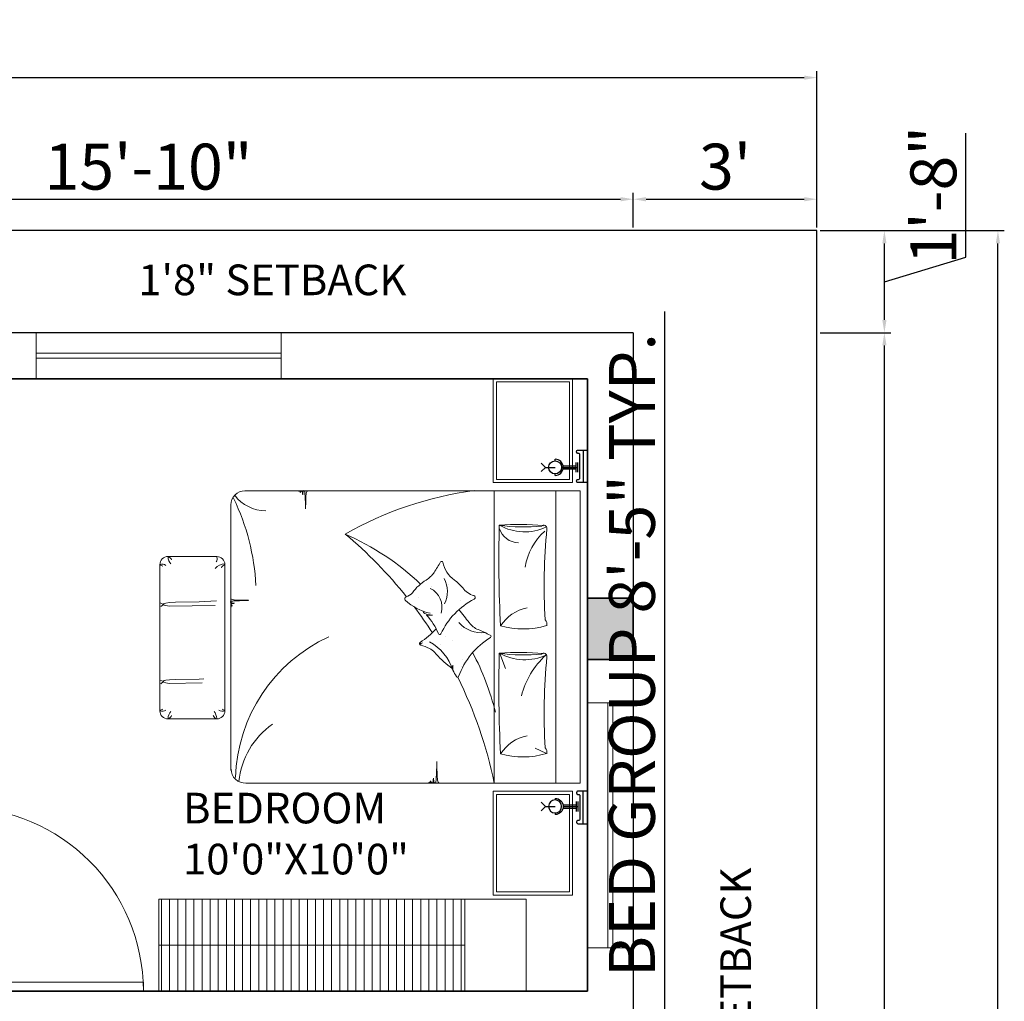
# Model space of a CAD drawing. Units: inches. Extents: x 3321 to 5237, y 11 to 1752.
# Tile 43 of 43: x 5010 to 5203, y 1556 to 1749. Entities that reach past the tile are written whole.
import ezdxf

# ---------------------------------------------------------------- set-up
doc = ezdxf.new("R2010")
doc.units = ezdxf.units.IN
for name, color, linetype, lineweight in [('A-ANNO-DIMS', 2, 'Continuous', 18), ('A-ANNO-TEXT', 7, 'Continuous', 18), ('A-AREA-IDEN', 7, 'Continuous', 18), ('A-COLS', 1, 'Continuous', 35), ('A-DOOR', 4, 'Continuous', 18), ('A-FLOR-CASE', 8, 'Continuous', 18), ('A-FLOR-CASE-PATT', 8, 'Continuous', 13), ('A-FLOR-EDGE', 7, 'Continuous', 25), ('A-GLAZ', 5, 'Continuous', 18), ('A-WALL', 7, 'Continuous', 35), ('C-PROP', 7, 'Continuous', 30), ('FUR', 42, 'Continuous', 18)]:
    doc.layers.add(name, color=color, linetype=linetype, lineweight=lineweight)
for name, color, linetype in [('CEIL', 4, 'Continuous'), ('ELEC', 4, 'Continuous'), ('wood', 26, 'Continuous')]:
    doc.layers.add(name, color=color, linetype=linetype)
doc.styles.get("Standard").update_dxf_attribs({"font": 'arial.ttf'})
doc.dimstyles.new('ISO-25', dxfattribs={"dimtxt": 9, "dimasz": 2.5, "dimexe": 1.25, "dimexo": 0.625, "dimtad": 1, "dimdec": 1, "dimlunit": 3, "dimtxsty": 'Standard', "dimcen": 2.5, "dimclrd": 4, "dimclre": 4, "dimclrt": 256, "dimadec": 0, "dimazin": 0, "dimtfac": 1, "dimtdec": 1, "dimtmove": 0, "dimatfit": 3, "dimfxl": 1, "dimarcsym": 0})

# ---------------------------------------------------------------- blocks, each defined once
blk = doc.blocks.new('*U4')
for p, q in [((0, 0), (0, -6)), ((-36, 0), (-36, -6))]:
    blk.add_line(p, q)
blk.add_lwpolyline([(0, 0), (0, 36), (-1.75, 36), (-1.75, 0)], close=True)
blk.add_arc((0, 0), 36, 90, 180)
blk = doc.blocks.new('*D14')
at = {"layer": 'A-ANNO-DIMS', "color": 0, "lineweight": -2, "transparency": 16777216}
for p, q in [((4940.08, 1707.96), (4940.08, 1714.75)), ((4942.58, 1713.5), (5127.58, 1713.5)), ((5130.08, 1707.96), (5130.08, 1714.75))]:
    blk.add_line(p, q, dxfattribs=at)
at = {"layer": 'A-ANNO-DIMS', "color": 0, "transparency": 16777216}
for points in [[(4942.58, 1713.92), (4942.58, 1713.08), (4940.08, 1713.5)], [(5127.58, 1713.92), (5127.58, 1713.08), (5130.08, 1713.5)]]:
    blk.add_solid(points, dxfattribs=at)
at = {"layer": 'Defpoints', "color": 0, "transparency": 16777216}
for p in [(5130.08, 1713.5), (4940.08, 1707.34), (5130.08, 1707.34)]:
    blk.add_point(p, dxfattribs=at)
at = {"layer": 'A-ANNO-DIMS', "color": 0, "transparency": 16777216, "insert": (5035.08, 1718.72), "char_height": 9, "attachment_point": 5}
blk.add_mtext('15\'-10"', dxfattribs=at)
blk = doc.blocks.new('*D15')
at = {"layer": 'A-ANNO-DIMS', "color": 0, "lineweight": -2, "transparency": 16777216}
for p, q in [((5130.08, 1707.96), (5130.08, 1714.75)), ((5132.58, 1713.5), (5163.58, 1713.5)), ((5166.08, 1707.96), (5166.08, 1714.75))]:
    blk.add_line(p, q, dxfattribs=at)
at = {"layer": 'A-ANNO-DIMS', "color": 0, "transparency": 16777216}
for points in [[(5132.58, 1713.92), (5132.58, 1713.08), (5130.08, 1713.5)], [(5163.58, 1713.92), (5163.58, 1713.08), (5166.08, 1713.5)]]:
    blk.add_solid(points, dxfattribs=at)
at = {"layer": 'Defpoints', "color": 0, "transparency": 16777216}
for p in [(5166.08, 1713.5), (5130.08, 1707.34), (5166.08, 1707.34)]:
    blk.add_point(p, dxfattribs=at)
at = {"layer": 'A-ANNO-DIMS', "color": 0, "transparency": 16777216, "insert": (5148.08, 1718.72), "char_height": 9, "attachment_point": 5}
blk.add_mtext("3'", dxfattribs=at)
blk = doc.blocks.new('*D22')
at = {"layer": 'A-ANNO-DIMS', "color": 0, "lineweight": -2, "transparency": 16777216}
for p, q in [((5166.71, 1687.34), (5180.54, 1687.34)), ((5179.29, 1339.84), (5179.29, 1684.84)), ((5166.71, 1337.34), (5180.54, 1337.34))]:
    blk.add_line(p, q, dxfattribs=at)
at = {"layer": 'A-ANNO-DIMS', "color": 0, "transparency": 16777216}
for points in [[(5178.88, 1684.84), (5179.71, 1684.84), (5179.29, 1687.34)], [(5178.88, 1339.84), (5179.71, 1339.84), (5179.29, 1337.34)]]:
    blk.add_solid(points, dxfattribs=at)
at = {"layer": 'Defpoints', "color": 0, "transparency": 16777216}
for p in [(5166.08, 1687.34), (5179.29, 1687.34), (5166.08, 1337.34)]:
    blk.add_point(p, dxfattribs=at)
at = {"layer": 'A-ANNO-DIMS', "color": 0, "transparency": 16777216, "insert": (5174.07, 1512.34), "char_height": 9, "attachment_point": 5, "rotation": 90}
blk.add_mtext('29\'-2"', dxfattribs=at)
blk = doc.blocks.new('*D23')
at = {"layer": 'A-ANNO-DIMS', "color": 0, "lineweight": -2, "transparency": 16777216}
for p, q in [((5195.27, 1702.13), (5195.27, 1726.46)), ((5166.71, 1707.34), (5180.54, 1707.34)), ((5179.29, 1689.84), (5179.29, 1704.84)), ((5179.29, 1697.34), (5195.27, 1702.13)), ((5166.71, 1687.34), (5180.54, 1687.34))]:
    blk.add_line(p, q, dxfattribs=at)
at = {"layer": 'A-ANNO-DIMS', "color": 0, "transparency": 16777216}
for points in [[(5178.88, 1704.84), (5179.71, 1704.84), (5179.29, 1707.34)], [(5178.88, 1689.84), (5179.71, 1689.84), (5179.29, 1687.34)]]:
    blk.add_solid(points, dxfattribs=at)
at = {"layer": 'Defpoints', "color": 0, "transparency": 16777216}
for p in [(5166.08, 1707.34), (5179.29, 1707.34), (5166.08, 1687.34)]:
    blk.add_point(p, dxfattribs=at)
at = {"layer": 'A-ANNO-DIMS', "color": 0, "transparency": 16777216, "insert": (5190.05, 1714.29), "char_height": 9, "attachment_point": 5, "rotation": 90}
blk.add_mtext('1\'-8"', dxfattribs=at)
blk = doc.blocks.new('*X127')
at = {"color": 0}
for p, q in [((3147.8, 8143.4), (3147.8, 8143.4)), ((3155.9, 8182.9), (3155.9, 8182.9)), ((3209.5, 8023.9), (3209.5, 8023.9)), ((3283, 8049.6), (3283, 8049.6)), ((3154.1, 7950.7), (3154.1, 7950.7)), ((3251.6, 7997), (3251.6, 7997))]:
    blk.add_line(p, q, dxfattribs=at)
blk = doc.blocks.new('*X126')
at = {"color": 0}
for p, q in [((3155.9, 8182.9), (3155.9, 8182.9)), ((3139.8, 7939.7), (3139.8, 7939.7))]:
    blk.add_line(p, q, dxfattribs=at)
blk = doc.blocks.new('*X125')
at = {"color": 0}
for p, q in [((3155.9, 8182.9), (3155.9, 8182.9)), ((3139.8, 7939.7), (3139.8, 7939.7))]:
    blk.add_line(p, q, dxfattribs=at)
blk = doc.blocks.new('*X124')
at = {"color": 0}
for p, q in [((3163, 7776.2), (3163, 7776.2)), ((3422.2, 7761.3), (3422.2, 7761.3)), ((3236.2, 7675.7), (3236.2, 7675.7)), ((3244.3, 7698.6), (3244.3, 7698.6)), ((3340.3, 7689.4), (3340.3, 7689.4))]:
    blk.add_line(p, q, dxfattribs=at)
blk = doc.blocks.new('BED1')
for p, q in [((0, -1000), (0, 800)), ((150, 800), (0, 800)), ((150, 800), (150, -1000)), ((2058.7, 800), (150, 800)), ((528, 800), (528, -1000)), ((211.8, 614.9), (277.5, 585.4)), ((2537.2, 404.9), (2237.2, 404.9)), ((2187.2, 354.9), (2187.2, -545.1)), ((2587.2, -545.1), (2587.2, 354.9)), ((2582, 188.1), (2565.4, 174.8)), ((2566.3, 178.5), (2565.2, 177.4)), ((2565.4, 174.8), (2585.7, 165.4)), ((2566.3, -296.8), (2565.2, -297.9)), ((2582, -287.1), (2565.4, -300.5)), ((2565.4, -300.5), (2585.7, -309.9)), ((2237.2, -595.1), (2537.2, -595.1)), ((150, -1000), (0, -1000)), ((150, -1000), (2063.5, -1000))]:
    blk.add_line(p, q)
for points in [[(934, 797.9), (930.9, 797.7), (928.3, 797.4), (926.3, 796.9), (924.9, 796.3), (923.8, 795.6), (923.1, 794.8), (922.7, 793.8), (922.5, 792.7), (922.4, 791.5), (922.5, 790.3), (922.6, 789.2), (922.6, 788.3), (922.6, 787.6), (922.4, 787.3), (922, 787.4), (921.4, 787.9), (920.6, 788.9), (919.5, 790.2), (918.4, 791.6), (917.1, 793.1), (915.9, 794.6), (914.6, 796), (913.3, 797.1), (912.2, 797.9), (911.1, 798.3), (910.1, 798.4), (909.2, 798), (908.3, 797.1), (907.5, 795.8), (906.8, 793.9), (906, 791.4), (905.4, 788.5), (904.8, 785.2), (904.2, 781.7), (903.7, 778.4), (903.2, 775.4), (902.8, 772.9), (902.5, 771.3), (902.3, 770.6), (902.1, 771.2), (902, 772.8), (901.8, 775.2), (901.7, 778.1), (901.5, 781.5), (901.2, 785), (900.8, 788.4), (900.2, 791.5), (899.5, 794.1), (898.6, 796.2), (897.6, 797.9), (896.5, 799.2), (895.3, 800), (894.1, 800.5), (893, 800.7), (891.9, 800.5), (890.9, 800.1), (890, 799), (889.1, 797.1), (888.3, 794), (887.6, 789.3), (886.9, 782.9), (886.2, 774.2), (885.5, 763.1), (884.8, 749.5), (884.2, 734.2), (883.6, 718.3), (883, 702.8), (882.5, 688.8), (882, 677.5), (881.7, 669.8), (881.5, 666.9), (881.3, 669.4), (881.3, 676.7), (881.3, 687.8), (881.2, 701.5), (881.1, 716.8), (880.8, 732.6), (880.2, 748), (879.4, 761.8), (878.3, 773.2), (876.9, 782.2), (875.1, 789.2), (872.9, 794.4), (870.3, 798), (869, 799)], [(2150, -913.5), (2150, 723.2)], [(2327.6, 182.3), (2530, 185.9), (2550.8, 181.9), (2561.7, 179), (2566, 176.7), (2566.9, 174.4), (2566.3, 171.9), (2562, 169.2), (2550.3, 166.5), (2527.7, 163.9), (2490.6, 161.8), (2345.5, 160.2), (2317.8, 158.5)], [(494.7, 3.1), (458.9, 95.3)], [(2149.7, -259.9), (2150, -268.4), (2150.1, -274.1), (2150.1, -278.1), (2150, -281.4), (2149.8, -284), (2149.5, -286.1), (2149.1, -287.8), (2148.7, -289), (2148.1, -289.9), (2147.4, -290.5), (2146.6, -290.8), (2145.6, -291), (2144.6, -291), (2143.6, -291), (2142.7, -290.9), (2141.9, -290.9), (2141.4, -290.9), (2141.1, -291), (2141.2, -291.4), (2141.7, -291.9), (2142.5, -292.6), (2143.5, -293.4), (2144.7, -294.4), (2146, -295.4), (2147.2, -296.5), (2148.4, -297.6), (2149.3, -298.6), (2150, -299.6), (2150.3, -300.5), (2150.4, -301.3), (2150, -302.1), (2149.3, -302.8), (2148.2, -303.5), (2146.6, -304.1), (2144.6, -304.7), (2142.1, -305.2), (2139.3, -305.7), (2136.5, -306.2), (2133.7, -306.6), (2131.2, -307), (2129.2, -307.3), (2127.8, -307.6), (2127.3, -307.8), (2127.7, -308), (2129, -308.1), (2131, -308.2), (2133.5, -308.3), (2136.3, -308.5), (2139.2, -308.7), (2142, -309), (2144.6, -309.5), (2146.8, -310.1), (2148.6, -310.9), (2150, -311.7), (2151, -312.7), (2151.7, -313.6), (2152.1, -314.6), (2152.3, -315.6), (2152.2, -316.5), (2151.8, -317.3), (2150.9, -318.1), (2149.3, -318.8), (2146.7, -319.4), (2142.8, -320), (2137.4, -320.6), (2130.2, -321.2), (2121, -321.8), (2109.7, -322.3), (2096.9, -322.9), (2083.6, -323.4), (2070.7, -323.9), (2059.1, -324.3), (2049.6, -324.7), (2043.2, -325), (2040.8, -325.2), (2042.9, -325.3), (2049, -325.3), (2058.2, -325.3), (2069.6, -325.4), (2082.3, -325.5), (2095.6, -325.8), (2108.4, -326.2), (2119.9, -326.8), (2129.4, -327.8), (2136.9, -329), (2142.7, -330.5), (2147, -332.3), (2150, -334.4), (2150.9, -335.6)], [(2246.5, -294.4), (2530, -289.4), (2550.8, -293.4), (2561.7, -296.3), (2566, -298.6), (2566.9, -300.8), (2566.3, -303.4), (2562, -306.1), (2550.3, -308.8), (2527.7, -311.3), (2490.6, -313.5), (2345.5, -315), (2238.6, -321.8)], [(1733.7, -998.3), (1731.1, -998.1), (1729, -997.8), (1727.4, -997.4), (1726.1, -997), (1725.2, -996.4), (1724.7, -995.7), (1724.3, -994.8), (1724.1, -993.9), (1724.1, -992.9), (1724.1, -991.9), (1724.2, -991), (1724.2, -990.2), (1724.2, -989.7), (1724.1, -989.4), (1723.8, -989.5), (1723.2, -990), (1722.5, -990.8), (1721.7, -991.8), (1720.7, -993), (1719.7, -994.3), (1718.6, -995.5), (1717.5, -996.6), (1716.5, -997.6), (1715.5, -998.3), (1714.6, -998.6), (1713.8, -998.6), (1713, -998.3), (1712.3, -997.6), (1711.7, -996.5), (1711, -994.9), (1710.4, -992.9), (1709.9, -990.4), (1709.4, -987.6), (1708.9, -984.8), (1708.5, -982), (1708.1, -979.5), (1707.8, -977.4), (1707.5, -976.1), (1707.3, -975.5), (1707.1, -976), (1707, -977.3), (1706.9, -979.3), (1706.8, -981.8), (1706.7, -984.6), (1706.4, -987.5), (1706.1, -990.3), (1705.6, -992.9), (1705, -995.1), (1704.2, -996.9), (1703.4, -998.3), (1702.4, -999.3), (1701.5, -1000), (1700.5, -1000.4), (1699.6, -1000.6), (1698.7, -1000.4), (1697.8, -1000.1), (1697, -999.2), (1696.3, -997.6), (1695.7, -995), (1695.1, -991.1), (1694.5, -985.7), (1693.9, -978.5), (1693.3, -969.3), (1692.8, -957.9), (1692.2, -945.2), (1691.7, -931.9), (1691.2, -919), (1690.8, -907.4), (1690.4, -897.9), (1690.1, -891.5), (1689.9, -889.1), (1689.8, -891.2), (1689.8, -897.3), (1689.8, -906.5), (1689.7, -917.9), (1689.6, -930.6), (1689.4, -943.8), (1688.9, -956.6), (1688.3, -968.1), (1687.3, -977.6), (1686.1, -985.2), (1684.6, -991), (1682.8, -995.3), (1680.7, -998.3), (1679.6, -999.2)]]:
    blk.add_lwpolyline(points)
for points in [[(205.5, 619.6, 0.267769), (215.1, 582.4, -0.037739), (204.3, 21.8, 0.684696), (236.7, 5.5, -0.060702), (497.2, 0.1, -0.046649), (225.9, 3.1, -1.318436)], [(489.2, 619.6, 0.144019), (207.6, 617.9, 0.248643)], [(497.2, 0.1, 0.021276), (489.2, 619.6, -0.206383), (326.6, 509.4, 0.237198)], [(211.8, 12.8, 0.143972), (361.6, 262.9, 1.292232)], [(886.4, -150, -0.069098), (985, -66.5, 0.658965), (982.1, -48.7, -0.049789), (927.4, -29, -0.103757), (896.6, -5.4, 0.055725), (800.9, 83.3, -0.11866), (782.7, 104.9, 0.016811), (761.6, 143.9, 0.70791), (748.3, 144, -0.16964), (551.9, -96.6, 0.664036), (554, -110.7, 0.023706), (627, -144.7, -0.134834), (683.2, -188, 0.012748), (746.3, -267.4)], [(969.1, -259.1, 0.263265), (936.3, -236.9, -0.026108), (909.2, -233.2, 0.027613), (945.1, -234.2, -0.089259), (872.7, -120, 0.662242), (857.6, -119.3, -0.162037), (651.8, -332.7, 0.676499), (654, -354.5, -0.160513), (722.9, -401.5, 0.07473), (773.5, -450.3, -0.187721), (845.5, -559.9, 0.70791), (858.8, -561.4, -0.010003), (898.6, -497.3, -0.113819), (947.3, -450.2, 0.099539), (1032.5, -372.4, -0.173425), (1070.9, -346.4, 0.589988), (1076.2, -326.1, 0.137312), (923.9, -245.9, 0.137312)], [(205.5, -168.2, 0.267769), (215.1, -205.4, -0.037739), (204.3, -766, 0.684696), (236.7, -782.3, -0.060702), (497.2, -787.7, -0.046649), (225.9, -784.7, -1.318436)], [(489.2, -168.2, 0.144019), (207.6, -169.9, 0.248643)], [(497.2, -787.7, 0.021276), (489.2, -168.2, -0.206383), (326.6, -278.4, 0.237198)], [(1446, -733.4, -0.095039), (652.8, -1001.7)]]:
    blk.add_lwpolyline(points, format="xyb")
for centre, radius, start, end in [((3208.8, 1363.3), 2739.4, 191.86791, 206.32469), ((1608.1, 842.5), 496.3, 305.19014, 354.02057), ((2062.7, 713.7), 86.5, 0, 93.53765), ((1138.6, 793.9), 983.2, 294.60777, 358.30329), ((2098.7, 754.7), 1625, 193.90497, 207.81692), ((2237.2, 354.9), 50, 90, 180), ((2321.1, 409.7), 84.5, 185.61958, 217.13957), ((2227.5, 373.5), 32.8, 17.83305, 72.80048), ((2546.9, 373.5), 32.8, 107.19952, 162.16695), ((2453.3, 409.7), 84.5, 322.86043, 354.38042), ((2537.2, 354.9), 50, 0, 90), ((2201.9, 323.3), 34.8, 50.8413, 114.9586), ((2212.2, 381.5), 36.5, 226.80948, 258.3841), ((2572.5, 323.3), 34.8, 65.0414, 129.1587), ((2562.2, 381.5), 36.5, 281.6159, 313.19052), ((751.8, 88.7), 34.9, 336.83517, 27.72181), ((684.2, 86), 100.3, 353.675, 10.88198), ((1074.1, 198.8), 306.1, 197.86019, 241.51221), ((341.4, -277.7), 318.5, 60.71255, 115.00895), ((983.7, -79.5), 20.8, 73.79673, 130.45661), ((978.5, -68.6), 14.3, 39.7097, 85.9506), ((602.5, -324), 198.6, 43.20348, 95.05559), ((3208.8, 1363.3), 2739.4, 212.93136, 216.95099), ((981.1, -281.8), 131.1, 164.0372, 243.45361), ((980, -379), 163.4, 152.61037, 209.36102), ((3208.8, 1363.3), 2739.4, 218.63292, 229.94485), ((3402.5, -342.9), 1408.5, 182.99169, 205.68187), ((2098.7, 754.7), 1625, 226.58872, 246.3156), ((-34.4, -471.2), 376.5, 312.01178, 350.96348), ((2178, -513.5), 33, 286.18268, 338.13858), ((2237.2, -545.1), 50, 180, 270), ((2188.1, -476.2), 73, 269.45125, 322.80265), ((2537.2, -545.1), 50, 270, 0), ((2572.5, -513.6), 34.8, 230.8413, 294.9586), ((2562.2, -571.8), 36.5, 46.80948, 78.3841), ((2271.1, -580.9), 35.8, 148.90546, 197.55407), ((2546.9, -563.8), 32.8, 197.83305, 252.80048), ((2453.3, -600), 84.5, 5.61958, 37.13957), ((375.7, -807.4), 128.2, 17.40732, 88.51286), ((341.4, -1065.5), 318.5, 60.71255, 115.00895), ((1929.1, -1126), 250.5, 37.85533, 88.44053), ((2063.5, -913.5), 86.5, 270, 0)]:
    blk.add_arc(centre, radius, start, end)
for name in ['*X126', '*X125', '*X127', '*X124']:
    blk.add_blockref(name, (-2425.3, -8101.4))
blk = doc.blocks.new('APLIQ')
at = {"layer": 'ELEC'}
for p, q in [((0, 0.2), (-0.0261, 0.2261)), ((0, 0.2), (0.0261, 0.2261)), ((0, 0.2), (0, 0.14)), ((-0.05, 0.14), (-0.04, 0.14)), ((0.04, 0.14), (0.05, 0.14)), ((-0.01, 0.09), (-0.01, 0.01)), ((0, 0.09), (0, 0)), ((0.01, 0.09), (0.01, 0.01)), ((-0.03, 0.01), (0.03, 0.01)), ((-0.03, 0), (0.03, 0))]:
    blk.add_line(p, q, dxfattribs=at)
blk.add_circle((0, 0.14), 0.04, dxfattribs=at)
blk.add_arc((0, 0.14), 0.05, 180, 0, dxfattribs=at)
blk = doc.blocks.new('A$C68AE1801')
at = {"layer": 'FUR'}
for points in [[(2.5416, 3.18), (2.5416, 2.54), (2.0516, 2.54), (2.0516, 3.18)], [(2.5216, 3.16), (2.5216, 2.56), (2.0716, 2.56), (2.0716, 3.16)], [(2.5416, 0), (2.5416, 0.64), (2.0516, 0.64), (2.0516, 0)], [(2.5216, 0.02), (2.5216, 0.62), (2.0716, 0.62), (2.0716, 0.02)]]:
    blk.add_lwpolyline(points, close=True, dxfattribs=at)
at = {"layer": 'wood'}
for p, q in [((2.6057, 2.74), (2.6057, 2.54)), ((2.6057, 0.44), (2.6057, 0.64))]:
    blk.add_line(p, q, dxfattribs=at)
for points in [[(2.5657, 2.728), (2.5657, 2.732, -0.414214), (2.5737, 2.74), (2.6321, 2.74), (2.6321, 2.54), (2.5737, 2.54, -0.414214), (2.5657, 2.548), (2.5657, 2.552, -0.414214), (2.5737, 2.56), (2.5777, 2.56, 0.414214), (2.5857, 2.568), (2.5857, 2.712, 0.414214), (2.5777, 2.72), (2.5737, 2.72, -0.414214)], [(2.5657, 0.452), (2.5657, 0.448, 0.414214), (2.5737, 0.44), (2.6321, 0.44), (2.6321, 0.64), (2.5737, 0.64, 0.414214), (2.5657, 0.632), (2.5657, 0.628, 0.414214), (2.5737, 0.62), (2.5777, 0.62, -0.414214), (2.5857, 0.612), (2.5857, 0.468, -0.414214), (2.5777, 0.46), (2.5737, 0.46, 0.414214)]]:
    blk.add_lwpolyline(points, format="xyb", close=True, dxfattribs=at)
at = {"layer": 'CEIL', "rotation": 90}
blk.add_blockref('APLIQ', (2.5736, 2.634), dxfattribs=at)
at = {"layer": 'CEIL', "xscale": -1, "rotation": 90}
blk.add_blockref('APLIQ', (2.5736, 0.546), dxfattribs=at)
at = {"layer": 'FUR', "xscale": 0.001, "yscale": 0.001, "zscale": 0.001, "rotation": 180}
blk.add_blockref('BED1', (2.5872, 1.49), dxfattribs=at)
blk = doc.blocks.new('*D148')
at = {"layer": 'A-ANNO-DIMS', "color": 0, "lineweight": -2, "transparency": 16777216}
for p, q in [((5166.71, 1707.34), (5202.79, 1707.34)), ((5201.54, 989.84), (5201.54, 1704.84)), ((5166.71, 987.34), (5202.79, 987.34))]:
    blk.add_line(p, q, dxfattribs=at)
at = {"layer": 'A-ANNO-DIMS', "color": 0, "transparency": 16777216}
for points in [[(5201.12, 1704.84), (5201.96, 1704.84), (5201.54, 1707.34)], [(5201.12, 989.84), (5201.96, 989.84), (5201.54, 987.34)]]:
    blk.add_solid(points, dxfattribs=at)
at = {"layer": 'Defpoints', "color": 0, "transparency": 16777216}
for p in [(5166.08, 1707.34), (5201.54, 1707.34), (5166.08, 987.34)]:
    blk.add_point(p, dxfattribs=at)
at = {"layer": 'A-ANNO-DIMS', "color": 0, "transparency": 16777216, "insert": (5196.32, 1347.34), "char_height": 9, "attachment_point": 5, "rotation": 90}
blk.add_mtext("60'", dxfattribs=at)
blk = doc.blocks.new('*D149')
at = {"layer": 'A-ANNO-DIMS', "color": 0, "lineweight": -2, "transparency": 16777216}
for p, q in [((4686.08, 1707.96), (4686.08, 1738.58)), ((5166.08, 1707.96), (5166.08, 1738.58)), ((4688.58, 1737.33), (5163.58, 1737.33))]:
    blk.add_line(p, q, dxfattribs=at)
at = {"layer": 'A-ANNO-DIMS', "color": 0, "transparency": 16777216}
for points in [[(4688.58, 1737.74), (4688.58, 1736.91), (4686.08, 1737.33)], [(5163.58, 1737.74), (5163.58, 1736.91), (5166.08, 1737.33)]]:
    blk.add_solid(points, dxfattribs=at)
at = {"layer": 'Defpoints', "color": 0, "transparency": 16777216}
for p in [(5166.08, 1737.33), (4686.08, 1707.34), (5166.08, 1707.34)]:
    blk.add_point(p, dxfattribs=at)
at = {"layer": 'A-ANNO-DIMS', "color": 0, "transparency": 16777216, "insert": (4926.08, 1742.55), "char_height": 9, "attachment_point": 5}
blk.add_mtext("40'", dxfattribs=at)
blk = doc.blocks.new('COL-9X12-FURN-PLAN')
h = blk.add_hatch(color=256)
h.dxf.hatch_style = 1
h.paths.add_polyline_path([(0, 12), (0, 0), (9, 0), (9, 12)])
blk.add_lwpolyline([(0, 0), (9, 0), (9, 12), (0, 12)], close=True)
blk = doc.blocks.new('WIN-48IN-9IN-WALL')
for p, q in [((0, 0), (0, 9)), ((48, 0), (48, 9)), ((0, 5), (48, 5)), ((0, 4), (48, 4))]:
    blk.add_line(p, q)
blk = doc.blocks.new('PROPERTY-40X60FT')
for p, q in [((0, 720), (0, 0)), ((0, 0), (480, 0))]:
    blk.add_line(p, q)
blk = doc.blocks.new('*D193')
at = {"layer": 'A-ANNO-DIMS', "color": 4, "lineweight": -2, "transparency": 16777216}
for p, q in [((5136.26, 1554.34), (5136.26, 1691.49)), ((5121.71, 1554.34), (5137.51, 1554.34)), ((5136.26, 1455.64), (5136.26, 1551.84)), ((5121.71, 1453.14), (5137.51, 1453.14))]:
    blk.add_line(p, q, dxfattribs=at)
at = {"layer": 'A-ANNO-DIMS', "color": 4, "transparency": 16777216}
for points in [[(5135.85, 1551.84), (5136.68, 1551.84), (5136.26, 1554.34)], [(5135.85, 1455.64), (5136.68, 1455.64), (5136.26, 1453.14)]]:
    blk.add_solid(points, dxfattribs=at)
at = {"layer": 'Defpoints', "color": 0, "transparency": 16777216}
for p in [(5121.08, 1554.34), (5136.26, 1554.34), (5121.08, 1453.14)]:
    blk.add_point(p, dxfattribs=at)
at = {"layer": 'A-ANNO-DIMS', "transparency": 16777216, "insert": (5130.98, 1624.17), "char_height": 9, "attachment_point": 5, "rotation": 90}
blk.add_mtext('BED GROUP 8\'-5" TYP.', dxfattribs=at)

msp = doc.modelspace()

# ---------------------------------------------------------------- hatches: boundary and pattern name
at = {"layer": 'A-FLOR-CASE-PATT'}
h = msp.add_hatch(dxfattribs=at)
h.set_pattern_fill('ANSI31', color=256, scale=0.5, angle=45)
h.set_pattern_definition([(90, (-1652.0904, 0), (-1.5875, 0), [])])
h.paths.add_polyline_path([(5097.08, 1576.34), (5037.08, 1576.34), (5037.08, 1567.34), (5097.08, 1567.34)])
h.paths.add_polyline_path([(5097.08, 1567.34), (5037.08, 1567.34), (5037.08, 1558.34), (5097.08, 1558.34)])

# ---------------------------------------------------------------- linework, layer by layer
at = {"layer": 'A-FLOR-CASE'}
for p, q in [((5109.08, 1576.34), (5037.08, 1576.34)), ((5037.08, 1576.34), (5037.08, 1558.34)), ((5097.08, 1576.34), (5097.08, 1558.34)), ((5109.08, 1576.34), (5109.08, 1558.34)), ((5037.08, 1567.34), (5097.08, 1567.34))]:
    msp.add_line(p, q, dxfattribs=at)
at = {"layer": 'A-FLOR-EDGE'}
for q in [(4731.08, 1687.34), (5130.08, 1091.34)]:
    msp.add_line((5130.08, 1687.34), q, dxfattribs=at)
at = {"layer": 'A-WALL'}
for p, q in [((5121.08, 1678.34), (5001.08, 1678.34)), ((5121.08, 1678.34), (5121.08, 1558.34)), ((5121.08, 1558.34), (4992.08, 1558.34))]:
    msp.add_line(p, q, dxfattribs=at)

# ---------------------------------------------------------------- block references
at = {"layer": 'A-COLS'}
msp.add_blockref('COL-9X12-FURN-PLAN', (5121.08, 1623.34), dxfattribs=at)
at = {"layer": 'A-DOOR', "rotation": 270}
msp.add_blockref('*U4', (4998.08, 1558.34), dxfattribs=at)
at = {"layer": 'A-GLAZ'}
msp.add_blockref('WIN-48IN-9IN-WALL', (5013.06, 1678.34), dxfattribs=at)
at = {"layer": 'A-GLAZ', "rotation": 90.00000000000031}
msp.add_blockref('WIN-48IN-9IN-WALL', (5130.08, 1566.84), dxfattribs=at)
at = {"layer": 'C-PROP', "rotation": 180}
msp.add_blockref('PROPERTY-40X60FT', (5166.08, 1707.34), dxfattribs=at)
at = {"layer": 'FUR', "xscale": 31.82298296329056, "yscale": 31.82298296329056, "zscale": 31.82298296329056}
msp.add_blockref('A$C68AE1801', (5037.32, 1577.14), dxfattribs=at)

# ---------------------------------------------------------------- texts
at = {"layer": 'A-ANNO-TEXT', "insert": (5033.07, 1700.7), "char_height": 6, "attachment_point": 1}
msp.add_mtext_dynamic_manual_height_columns('1\'8" SETBACK', width=97.3114, gutter_width=25, heights=[0], dxfattribs=at)
at = {"layer": 'A-ANNO-TEXT', "insert": (5147.15, 1530.01), "char_height": 6, "attachment_point": 1, "rotation": 90}
msp.add_mtext_dynamic_manual_height_columns('3\'0" SETBACK', width=97.3114, gutter_width=25, heights=[0], dxfattribs=at)
at = {"layer": 'A-AREA-IDEN', "insert": (5041.86, 1597.2), "char_height": 6, "attachment_point": 1}
msp.add_mtext_dynamic_manual_height_columns('BEDROOM\\P10\'0"X10\'0"', width=97.3114, gutter_width=25, heights=[0], dxfattribs=at)

# ---------------------------------------------------------------- dimensions: what is measured, and where the dimension line sits
at = {"layer": 'A-ANNO-DIMS'}
for base, p1, p2, picture, middle in [((5166.08, 1737.33), (4686.08, 1707.34), (5166.08, 1707.34), '*D149', (4926.08, 1742.55)), ((5130.08, 1713.5), (4940.08, 1707.34), (5130.08, 1707.34), '*D14', (5035.08, 1718.72)), ((5166.08, 1713.5), (5130.08, 1707.34), (5166.08, 1707.34), '*D15', (5148.08, 1718.72))]:
    dim = msp.add_linear_dim(base=base, p1=p1, p2=p2, dimstyle='ISO-25', override={"dimclrd": 0, "dimclre": 0, "dimclrt": 0}, dxfattribs=at)
    dim.commit()
    dim.dimension.update_dxf_attribs({"geometry": picture, "text_midpoint": middle})
for base, p1, p2, angle, override, picture, middle in [((5179.29, 1707.34), (5166.08, 1687.34), (5166.08, 1707.34), 90, {"dimclrd": 0, "dimclre": 0, "dimclrt": 0, "dimtmove": 1}, '*D23', (5190.05, 1702.76)), ((5201.54, 1707.34), (5166.08, 987.34), (5166.08, 1707.34), 270, {"dimclrd": 0, "dimclre": 0, "dimclrt": 0}, '*D148', (5196.32, 1347.34)), ((5179.29, 1687.34), (5166.08, 1337.34), (5166.08, 1687.34), 90, {"dimclrd": 0, "dimclre": 0, "dimclrt": 0, "dimtmove": 1}, '*D22', (5174.07, 1512.34))]:
    dim = msp.add_linear_dim(base=base, p1=p1, p2=p2, angle=angle, dimstyle='ISO-25', override=override, dxfattribs=at)
    dim.commit()
    dim.dimension.update_dxf_attribs({"geometry": picture, "text_midpoint": middle})
dim = msp.add_linear_dim(base=(5136.26, 1554.34), p1=(5121.08, 1453.14), p2=(5121.08, 1554.34), angle=90, text='BED GROUP <> TYP.', dimstyle='ISO-25', override={"dimdec": 1, "dimlfac": 1, "dimrnd": 0, "dimzin": 1, "dimdsep": 46, "dimlunit": 4, "dimfrac": 2}, dxfattribs=at)
dim.commit()
dim.dimension.update_dxf_attribs({"geometry": '*D193', "text_midpoint": (5130.98, 1624.17)})

doc.saveas('drawing.dxf')
